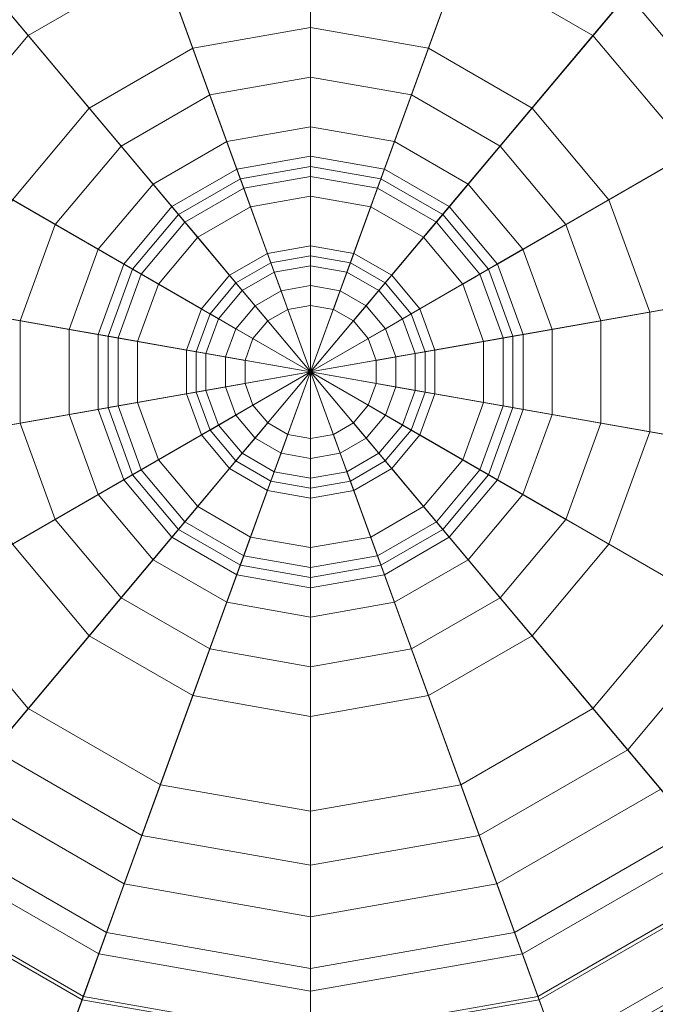
# Model space of a CAD drawing. Units: inches. Extents: x 375 to 1122, y 27 to 1069.
# Tile 129 of 155: x 721.601 to 722.65, y 901.45 to 903.075. Entities that reach past the tile are written whole.
import ezdxf

# ---------------------------------------------------------------- set-up
doc = ezdxf.new("R2010")
doc.units = ezdxf.units.IN
doc.layers.add('A-ANNO-DIMS', color=2, linetype='Continuous', lineweight=18)
doc.layers.add('Furniture', color=30, linetype='Continuous', lineweight=18)
doc.styles.get("Standard").update_dxf_attribs({"font": 'arial.ttf'})
doc.dimstyles.new('ISO-25', dxfattribs={"dimtxt": 12, "dimasz": 2.5, "dimexe": 1.5, "dimexo": 1.5, "dimtad": 1, "dimdec": 1, "dimlunit": 3, "dimtxsty": 'Standard', "dimblk": 'ARCHTICK', "dimcen": 2.5, "dimadec": 0, "dimazin": 0, "dimtfac": 1, "dimtdec": 1, "dimtmove": 0, "dimatfit": 3, "dimfxl": 1.5, "dimfxlon": 1, "dimarcsym": 0})

# ---------------------------------------------------------------- blocks, each defined once
blk = doc.blocks.new('A$C403C54AD')
for points in [[(0.889855, 0.961682, -0.042784), (0.895735, 0.928335, -0.039705), (0.895735, 0.928335, -0.039705), (0.878804, 0.95766, -0.042784)], [(0.901615, 0.961682, -0.042784), (0.895735, 0.928335, -0.039705), (0.895735, 0.928335, -0.039705), (0.889855, 0.961682, -0.042784)], [(0.912666, 0.95766, -0.042784), (0.895735, 0.928335, -0.039705), (0.895735, 0.928335, -0.039705), (0.901615, 0.961682, -0.042784)], [(0.893266, 0.942333, -0.036278), (0.890422, 0.958466, -0.039553), (0.880436, 0.954832, -0.039553), (0.888627, 0.940645, -0.036278)], [(0.898203, 0.942333, -0.036278), (0.901048, 0.958466, -0.039553), (0.890422, 0.958466, -0.039553), (0.893266, 0.942333, -0.036278)], [(0.902842, 0.940645, -0.036278), (0.911033, 0.954832, -0.039553), (0.901048, 0.958466, -0.039553), (0.898203, 0.942333, -0.036278)], [(0.878804, 0.95766, -0.042784), (0.895735, 0.928335, -0.039705), (0.895735, 0.928335, -0.039705), (0.869795, 0.950101, -0.042784)], [(0.921675, 0.950101, -0.042784), (0.895735, 0.928335, -0.039705), (0.895735, 0.928335, -0.039705), (0.912666, 0.95766, -0.042784)], [(0.888627, 0.940645, -0.036278), (0.880436, 0.954832, -0.039553), (0.872296, 0.948002, -0.039553), (0.884846, 0.937471, -0.036278)], [(0.906623, 0.937471, -0.036278), (0.919173, 0.948002, -0.039553), (0.911033, 0.954832, -0.039553), (0.902842, 0.940645, -0.036278)], [(0.882023, 0.952084, 0.060725), (0.885556, 0.945965, 0.050493), (0.88014, 0.94142, 0.050493), (0.874727, 0.945962, 0.060725)], [(0.916743, 0.945962, 0.060725), (0.911329, 0.94142, 0.050493), (0.905913, 0.945965, 0.050493), (0.909447, 0.952084, 0.060725)], [(0.869795, 0.950101, -0.042784), (0.895735, 0.928335, -0.039705), (0.895735, 0.928335, -0.039705), (0.863915, 0.939916, -0.042784)], [(0.927555, 0.939916, -0.042784), (0.895735, 0.928335, -0.039705), (0.895735, 0.928335, -0.039705), (0.921675, 0.950101, -0.042784)], [(0.924486, 0.938799, -0.039553), (0.927555, 0.939916, -0.042784), (0.921675, 0.950101, -0.042784), (0.919173, 0.948002, -0.039553)], [(0.886671, 0.944033, 0.05268), (0.883428, 0.94965, 0.062072), (0.87688, 0.944156, 0.062072), (0.881848, 0.939987, 0.05268)], [(0.909621, 0.939987, 0.05268), (0.914589, 0.944156, 0.062072), (0.908041, 0.94965, 0.062072), (0.904798, 0.944033, 0.05268)], [(0.924448, 0.938785, 0.1202), (0.92718, 0.93978, 0.106976), (0.921369, 0.949844, 0.106976), (0.919142, 0.947976, 0.1202)], [(0.92718, 0.93978, 0.106976), (0.926546, 0.939549, 0.078734), (0.920852, 0.949411, 0.078734), (0.921369, 0.949844, 0.106976)], [(0.926546, 0.939549, 0.078734), (0.921505, 0.937714, 0.060725), (0.916743, 0.945962, 0.060725), (0.920852, 0.949411, 0.078734)], [(0.884846, 0.937471, -0.036278), (0.872296, 0.948002, -0.039553), (0.866983, 0.938799, -0.039553), (0.882378, 0.933196, -0.036278)], [(0.8922, 0.948383, 0.050493), (0.893978, 0.9383, 0.043125), (0.890675, 0.937098, 0.043125), (0.885556, 0.945965, 0.050493)], [(0.89927, 0.948383, 0.050493), (0.897492, 0.9383, 0.043125), (0.893978, 0.9383, 0.043125), (0.8922, 0.948383, 0.050493)], [(0.905913, 0.945965, 0.050493), (0.900794, 0.937098, 0.043125), (0.897492, 0.9383, 0.043125), (0.89927, 0.948383, 0.050493)], [(0.909092, 0.933196, -0.036278), (0.924486, 0.938799, -0.039553), (0.919173, 0.948002, -0.039553), (0.906623, 0.937471, -0.036278)], [(0.919753, 0.937076, 0.129606), (0.924448, 0.938785, 0.1202), (0.919142, 0.947976, 0.1202), (0.915314, 0.944764, 0.129606)], [(0.924281, 0.938725, 0.106759), (0.921641, 0.937764, 0.119395), (0.916854, 0.946056, 0.119395), (0.919006, 0.947862, 0.106759)], [(0.923663, 0.9385, 0.079219), (0.924281, 0.938725, 0.106759), (0.919006, 0.947862, 0.106759), (0.918502, 0.947439, 0.079219)], [(0.918863, 0.936753, 0.062072), (0.923663, 0.9385, 0.079219), (0.918502, 0.947439, 0.079219), (0.914589, 0.944156, 0.062072)], [(0.894188, 0.937103, 0.046044), (0.892587, 0.946186, 0.05268), (0.886671, 0.944033, 0.05268), (0.891283, 0.936046, 0.046044)], [(0.897281, 0.937103, 0.046044), (0.898882, 0.946186, 0.05268), (0.892587, 0.946186, 0.05268), (0.894188, 0.937103, 0.046044)], [(0.900187, 0.936046, 0.046044), (0.904798, 0.944033, 0.05268), (0.898882, 0.946186, 0.05268), (0.897281, 0.937103, 0.046044)], [(0.921641, 0.937764, 0.119395), (0.91686, 0.936024, 0.129606), (0.912956, 0.942785, 0.129606), (0.916854, 0.946056, 0.119395)], [(0.885556, 0.945965, 0.050493), (0.890675, 0.937098, 0.043125), (0.887983, 0.934839, 0.043125), (0.88014, 0.94142, 0.050493)], [(0.911329, 0.94142, 0.050493), (0.903486, 0.934839, 0.043125), (0.900794, 0.937098, 0.043125), (0.905913, 0.945965, 0.050493)], [(0.921505, 0.937714, 0.060725), (0.914864, 0.935297, 0.050493), (0.911329, 0.94142, 0.050493), (0.916743, 0.945962, 0.060725)], [(0.91686, 0.936024, 0.129606), (0.919753, 0.937076, 0.129606), (0.915314, 0.944764, 0.129606), (0.912956, 0.942785, 0.129606)], [(0.881848, 0.939987, 0.05268), (0.87688, 0.944156, 0.062072), (0.872606, 0.936753, 0.062072), (0.878701, 0.934534, 0.05268)], [(0.891283, 0.936046, 0.046044), (0.886671, 0.944033, 0.05268), (0.881848, 0.939987, 0.05268), (0.888914, 0.934058, 0.046044)], [(0.902556, 0.934058, 0.046044), (0.909621, 0.939987, 0.05268), (0.904798, 0.944033, 0.05268), (0.900187, 0.936046, 0.046044)], [(0.912769, 0.934534, 0.05268), (0.918863, 0.936753, 0.062072), (0.914589, 0.944156, 0.062072), (0.909621, 0.939987, 0.05268)], [(0.893622, 0.940316, -0.033413), (0.893266, 0.942333, -0.036278), (0.888627, 0.940645, -0.036278), (0.889651, 0.938871, -0.033413)], [(0.897847, 0.940316, -0.033413), (0.898203, 0.942333, -0.036278), (0.893266, 0.942333, -0.036278), (0.893622, 0.940316, -0.033413)], [(0.901818, 0.938871, -0.033413), (0.902842, 0.940645, -0.036278), (0.898203, 0.942333, -0.036278), (0.897847, 0.940316, -0.033413)], [(0.88014, 0.94142, 0.050493), (0.887983, 0.934839, 0.043125), (0.886226, 0.931795, 0.043125), (0.876605, 0.935297, 0.050493)], [(0.914864, 0.935297, 0.050493), (0.905243, 0.931795, 0.043125), (0.903486, 0.934839, 0.043125), (0.911329, 0.94142, 0.050493)], [(0.889651, 0.938871, -0.033413), (0.888627, 0.940645, -0.036278), (0.884846, 0.937471, -0.036278), (0.886415, 0.936155, -0.033413)], [(0.894333, 0.936283, -0.031367), (0.893622, 0.940316, -0.033413), (0.889651, 0.938871, -0.033413), (0.891699, 0.935324, -0.031367)], [(0.897136, 0.936283, -0.031367), (0.897847, 0.940316, -0.033413), (0.893622, 0.940316, -0.033413), (0.894333, 0.936283, -0.031367)], [(0.89977, 0.935324, -0.031367), (0.901818, 0.938871, -0.033413), (0.897847, 0.940316, -0.033413), (0.897136, 0.936283, -0.031367)], [(0.905055, 0.936155, -0.033413), (0.906623, 0.937471, -0.036278), (0.902842, 0.940645, -0.036278), (0.901818, 0.938871, -0.033413)], [(0.863915, 0.939916, -0.042784), (0.895735, 0.928335, -0.039705), (0.895735, 0.928335, -0.039705), (0.861872, 0.928335, -0.042784)], [(0.888914, 0.934058, 0.046044), (0.881848, 0.939987, 0.05268), (0.878701, 0.934534, 0.05268), (0.887368, 0.93138, 0.046044)], [(0.929597, 0.928335, -0.042784), (0.895735, 0.928335, -0.039705), (0.895735, 0.928335, -0.039705), (0.927555, 0.939916, -0.042784)], [(0.904102, 0.93138, 0.046044), (0.912769, 0.934534, 0.05268), (0.909621, 0.939987, 0.05268), (0.902556, 0.934058, 0.046044)], [(0.928523, 0.928335, 0.078734), (0.923158, 0.928335, 0.060725), (0.921505, 0.937714, 0.060725), (0.926546, 0.939549, 0.078734)], [(0.882378, 0.933196, -0.036278), (0.866983, 0.938799, -0.039553), (0.865138, 0.928335, -0.039553), (0.88152, 0.928335, -0.036278)], [(0.891699, 0.935324, -0.031367), (0.889651, 0.938871, -0.033413), (0.886415, 0.936155, -0.033413), (0.889552, 0.933523, -0.031367)], [(0.901917, 0.933523, -0.031367), (0.905055, 0.936155, -0.033413), (0.901818, 0.938871, -0.033413), (0.89977, 0.935324, -0.031367)], [(0.909949, 0.928335, -0.036278), (0.926331, 0.928335, -0.039553), (0.924486, 0.938799, -0.039553), (0.909092, 0.933196, -0.036278)], [(0.921294, 0.928335, 0.129606), (0.926291, 0.928335, 0.1202), (0.924448, 0.938785, 0.1202), (0.919753, 0.937076, 0.129606)], [(0.926113, 0.928335, 0.106759), (0.923304, 0.928335, 0.119395), (0.921641, 0.937764, 0.119395), (0.924281, 0.938725, 0.106759)], [(0.893978, 0.9383, 0.043125), (0.894831, 0.93346, 0.042307), (0.893133, 0.932841, 0.042307), (0.890675, 0.937098, 0.043125)], [(0.897492, 0.9383, 0.043125), (0.896638, 0.93346, 0.042307), (0.894831, 0.93346, 0.042307), (0.893978, 0.9383, 0.043125)], [(0.900794, 0.937098, 0.043125), (0.898337, 0.932841, 0.042307), (0.896638, 0.93346, 0.042307), (0.897492, 0.9383, 0.043125)], [(0.920348, 0.928335, 0.062072), (0.925455, 0.928335, 0.079219), (0.923663, 0.9385, 0.079219), (0.918863, 0.936753, 0.062072)], [(0.886415, 0.936155, -0.033413), (0.884846, 0.937471, -0.036278), (0.882378, 0.933196, -0.036278), (0.884302, 0.932496, -0.033413)], [(0.907167, 0.932496, -0.033413), (0.909092, 0.933196, -0.036278), (0.906623, 0.937471, -0.036278), (0.905055, 0.936155, -0.033413)], [(0.923158, 0.928335, 0.060725), (0.916092, 0.928335, 0.050493), (0.914864, 0.935297, 0.050493), (0.921505, 0.937714, 0.060725)], [(0.923304, 0.928335, 0.119395), (0.918216, 0.928335, 0.129606), (0.91686, 0.936024, 0.129606), (0.921641, 0.937764, 0.119395)], [(0.890675, 0.937098, 0.043125), (0.893133, 0.932841, 0.042307), (0.891748, 0.93168, 0.042307), (0.887983, 0.934839, 0.043125)], [(0.895735, 0.928335, 0.044561), (0.894188, 0.937103, 0.046044), (0.891283, 0.936046, 0.046044), (0.895735, 0.928335, 0.044561)], [(0.895735, 0.928335, 0.044561), (0.897281, 0.937103, 0.046044), (0.894188, 0.937103, 0.046044), (0.895735, 0.928335, 0.044561)], [(0.895735, 0.928335, 0.044561), (0.900187, 0.936046, 0.046044), (0.897281, 0.937103, 0.046044), (0.895735, 0.928335, 0.044561)], [(0.903486, 0.934839, 0.043125), (0.899721, 0.93168, 0.042307), (0.898337, 0.932841, 0.042307), (0.900794, 0.937098, 0.043125)], [(0.918216, 0.928335, 0.129606), (0.921294, 0.928335, 0.129606), (0.919753, 0.937076, 0.129606), (0.91686, 0.936024, 0.129606)], [(0.894475, 0.935476, 0.041488), (0.894262, 0.936686, 0.039442), (0.891494, 0.935679, 0.039442), (0.892109, 0.934615, 0.041488)], [(0.894262, 0.936686, 0.039442), (0.894973, 0.932653, 0.037395), (0.893542, 0.932132, 0.037395), (0.891494, 0.935679, 0.039442)], [(0.896994, 0.935476, 0.041488), (0.897207, 0.936686, 0.039442), (0.894262, 0.936686, 0.039442), (0.894475, 0.935476, 0.041488)], [(0.897207, 0.936686, 0.039442), (0.896496, 0.932653, 0.037395), (0.894973, 0.932653, 0.037395), (0.894262, 0.936686, 0.039442)], [(0.899975, 0.935679, 0.039442), (0.897927, 0.932132, 0.037395), (0.896496, 0.932653, 0.037395), (0.897207, 0.936686, 0.039442)], [(0.899361, 0.934615, 0.041488), (0.899975, 0.935679, 0.039442), (0.897207, 0.936686, 0.039442), (0.896994, 0.935476, 0.041488)], [(0.913862, 0.928335, 0.05268), (0.920348, 0.928335, 0.062072), (0.918863, 0.936753, 0.062072), (0.912769, 0.934534, 0.05268)], [(0.894902, 0.933056, -0.026046), (0.894333, 0.936283, -0.031367), (0.891699, 0.935324, -0.031367), (0.893337, 0.932487, -0.026046)], [(0.896567, 0.933056, -0.026046), (0.897136, 0.936283, -0.031367), (0.894333, 0.936283, -0.031367), (0.894902, 0.933056, -0.026046)], [(0.898132, 0.932487, -0.026046), (0.89977, 0.935324, -0.031367), (0.897136, 0.936283, -0.031367), (0.896567, 0.933056, -0.026046)], [(0.889552, 0.933523, -0.031367), (0.886415, 0.936155, -0.033413), (0.884302, 0.932496, -0.033413), (0.88815, 0.931095, -0.031367)], [(0.895735, 0.928335, 0.044561), (0.891283, 0.936046, 0.046044), (0.888914, 0.934058, 0.046044), (0.895735, 0.928335, 0.044561)], [(0.895735, 0.928335, 0.044561), (0.902556, 0.934058, 0.046044), (0.900187, 0.936046, 0.046044), (0.895735, 0.928335, 0.044561)], [(0.903319, 0.931095, -0.031367), (0.907167, 0.932496, -0.033413), (0.905055, 0.936155, -0.033413), (0.901917, 0.933523, -0.031367)], [(0.891494, 0.935679, 0.039442), (0.893542, 0.932132, 0.037395), (0.892376, 0.931153, 0.037395), (0.889238, 0.933786, 0.039442)], [(0.892109, 0.934615, 0.041488), (0.891494, 0.935679, 0.039442), (0.889238, 0.933786, 0.039442), (0.890179, 0.932996, 0.041488)], [(0.894831, 0.93346, 0.042307), (0.894475, 0.935476, 0.041488), (0.892109, 0.934615, 0.041488), (0.893133, 0.932841, 0.042307)], [(0.896638, 0.93346, 0.042307), (0.896994, 0.935476, 0.041488), (0.894475, 0.935476, 0.041488), (0.894831, 0.93346, 0.042307)], [(0.898337, 0.932841, 0.042307), (0.899361, 0.934615, 0.041488), (0.896994, 0.935476, 0.041488), (0.896638, 0.93346, 0.042307)], [(0.902231, 0.933786, 0.039442), (0.899094, 0.931153, 0.037395), (0.897927, 0.932132, 0.037395), (0.899975, 0.935679, 0.039442)], [(0.90129, 0.932996, 0.041488), (0.902231, 0.933786, 0.039442), (0.899975, 0.935679, 0.039442), (0.899361, 0.934615, 0.041488)], [(0.876605, 0.935297, 0.050493), (0.886226, 0.931795, 0.043125), (0.885616, 0.928335, 0.043125), (0.875377, 0.928335, 0.050493)], [(0.893337, 0.932487, -0.026046), (0.891699, 0.935324, -0.031367), (0.889552, 0.933523, -0.031367), (0.892062, 0.931416, -0.026046)], [(0.899407, 0.931416, -0.026046), (0.901917, 0.933523, -0.031367), (0.89977, 0.935324, -0.031367), (0.898132, 0.932487, -0.026046)], [(0.916092, 0.928335, 0.050493), (0.905853, 0.928335, 0.043125), (0.905243, 0.931795, 0.043125), (0.914864, 0.935297, 0.050493)], [(0.887983, 0.934839, 0.043125), (0.891748, 0.93168, 0.042307), (0.890844, 0.930114, 0.042307), (0.886226, 0.931795, 0.043125)], [(0.893133, 0.932841, 0.042307), (0.892109, 0.934615, 0.041488), (0.890179, 0.932996, 0.041488), (0.891748, 0.93168, 0.042307)], [(0.899721, 0.93168, 0.042307), (0.90129, 0.932996, 0.041488), (0.899361, 0.934615, 0.041488), (0.898337, 0.932841, 0.042307)], [(0.905243, 0.931795, 0.043125), (0.900625, 0.930114, 0.042307), (0.899721, 0.93168, 0.042307), (0.903486, 0.934839, 0.043125)], [(0.887368, 0.93138, 0.046044), (0.878701, 0.934534, 0.05268), (0.877607, 0.928335, 0.05268), (0.886831, 0.928335, 0.046044)], [(0.904639, 0.928335, 0.046044), (0.913862, 0.928335, 0.05268), (0.912769, 0.934534, 0.05268), (0.904102, 0.93138, 0.046044)], [(0.895735, 0.928335, 0.044561), (0.888914, 0.934058, 0.046044), (0.887368, 0.93138, 0.046044), (0.895735, 0.928335, 0.044561)], [(0.889238, 0.933786, 0.039442), (0.892376, 0.931153, 0.037395), (0.891614, 0.929834, 0.037395), (0.887766, 0.931235, 0.039442)], [(0.890179, 0.932996, 0.041488), (0.889238, 0.933786, 0.039442), (0.887766, 0.931235, 0.039442), (0.88892, 0.930815, 0.041488)], [(0.895735, 0.928335, 0.044561), (0.904102, 0.93138, 0.046044), (0.902556, 0.934058, 0.046044), (0.895735, 0.928335, 0.044561)], [(0.903704, 0.931235, 0.039442), (0.899855, 0.929834, 0.037395), (0.899094, 0.931153, 0.037395), (0.902231, 0.933786, 0.039442)], [(0.902549, 0.930815, 0.041488), (0.903704, 0.931235, 0.039442), (0.902231, 0.933786, 0.039442), (0.90129, 0.932996, 0.041488)], [(0.892062, 0.931416, -0.026046), (0.889552, 0.933523, -0.031367), (0.88815, 0.931095, -0.031367), (0.891229, 0.929974, -0.026046)], [(0.90024, 0.929974, -0.026046), (0.903319, 0.931095, -0.031367), (0.901917, 0.933523, -0.031367), (0.899407, 0.931416, -0.026046)], [(0.884302, 0.932496, -0.033413), (0.882378, 0.933196, -0.036278), (0.88152, 0.928335, -0.036278), (0.883568, 0.928335, -0.033413)], [(0.891748, 0.93168, 0.042307), (0.890179, 0.932996, 0.041488), (0.88892, 0.930815, 0.041488), (0.890844, 0.930114, 0.042307)], [(0.895115, 0.931846, -0.017451), (0.894902, 0.933056, -0.026046), (0.893337, 0.932487, -0.026046), (0.893952, 0.931423, -0.017451)], [(0.896354, 0.931846, -0.017451), (0.896567, 0.933056, -0.026046), (0.894902, 0.933056, -0.026046), (0.895115, 0.931846, -0.017451)], [(0.897518, 0.931423, -0.017451), (0.898132, 0.932487, -0.026046), (0.896567, 0.933056, -0.026046), (0.896354, 0.931846, -0.017451)], [(0.900625, 0.930114, 0.042307), (0.902549, 0.930815, 0.041488), (0.90129, 0.932996, 0.041488), (0.899721, 0.93168, 0.042307)], [(0.907901, 0.928335, -0.033413), (0.909949, 0.928335, -0.036278), (0.909092, 0.933196, -0.036278), (0.907167, 0.932496, -0.033413)], [(0.894973, 0.932653, 0.037395), (0.895258, 0.93104, 0.030847), (0.894361, 0.930713, 0.030847), (0.893542, 0.932132, 0.037395)], [(0.896496, 0.932653, 0.037395), (0.896212, 0.93104, 0.030847), (0.895258, 0.93104, 0.030847), (0.894973, 0.932653, 0.037395)], [(0.897927, 0.932132, 0.037395), (0.897108, 0.930713, 0.030847), (0.896212, 0.93104, 0.030847), (0.896496, 0.932653, 0.037395)], [(0.88815, 0.931095, -0.031367), (0.884302, 0.932496, -0.033413), (0.883568, 0.928335, -0.033413), (0.887664, 0.928335, -0.031367)], [(0.893952, 0.931423, -0.017451), (0.893337, 0.932487, -0.026046), (0.892062, 0.931416, -0.026046), (0.893003, 0.930627, -0.017451)], [(0.898466, 0.930627, -0.017451), (0.899407, 0.931416, -0.026046), (0.898132, 0.932487, -0.026046), (0.897518, 0.931423, -0.017451)], [(0.903806, 0.928335, -0.031367), (0.907901, 0.928335, -0.033413), (0.907167, 0.932496, -0.033413), (0.903319, 0.931095, -0.031367)], [(0.886226, 0.931795, 0.043125), (0.890844, 0.930114, 0.042307), (0.890531, 0.928335, 0.042307), (0.885616, 0.928335, 0.043125)], [(0.893542, 0.932132, 0.037395), (0.894361, 0.930713, 0.030847), (0.89363, 0.9301, 0.030847), (0.892376, 0.931153, 0.037395)], [(0.895258, 0.93104, 0.030847), (0.895115, 0.931846, -0.017451), (0.893952, 0.931423, -0.017451), (0.894361, 0.930713, 0.030847)], [(0.896212, 0.93104, 0.030847), (0.896354, 0.931846, -0.017451), (0.895115, 0.931846, -0.017451), (0.895258, 0.93104, 0.030847)], [(0.897108, 0.930713, 0.030847), (0.897518, 0.931423, -0.017451), (0.896354, 0.931846, -0.017451), (0.896212, 0.93104, 0.030847)], [(0.899094, 0.931153, 0.037395), (0.897839, 0.9301, 0.030847), (0.897108, 0.930713, 0.030847), (0.897927, 0.932132, 0.037395)], [(0.905853, 0.928335, 0.043125), (0.900939, 0.928335, 0.042307), (0.900625, 0.930114, 0.042307), (0.905243, 0.931795, 0.043125)], [(0.895735, 0.928335, 0.044561), (0.887368, 0.93138, 0.046044), (0.886831, 0.928335, 0.046044), (0.895735, 0.928335, 0.044561)], [(0.893003, 0.930627, -0.017451), (0.892062, 0.931416, -0.026046), (0.891229, 0.929974, -0.026046), (0.892384, 0.929554, -0.017451)], [(0.894361, 0.930713, 0.030847), (0.893952, 0.931423, -0.017451), (0.893003, 0.930627, -0.017451), (0.89363, 0.9301, 0.030847)], [(0.895735, 0.928335, 0.044561), (0.904639, 0.928335, 0.046044), (0.904102, 0.93138, 0.046044), (0.895735, 0.928335, 0.044561)], [(0.897839, 0.9301, 0.030847), (0.898466, 0.930627, -0.017451), (0.897518, 0.931423, -0.017451), (0.897108, 0.930713, 0.030847)], [(0.899085, 0.929554, -0.017451), (0.90024, 0.929974, -0.026046), (0.899407, 0.931416, -0.026046), (0.898466, 0.930627, -0.017451)], [(0.887766, 0.931235, 0.039442), (0.891614, 0.929834, 0.037395), (0.89135, 0.928335, 0.037395), (0.887254, 0.928335, 0.039442)], [(0.88892, 0.930815, 0.041488), (0.887766, 0.931235, 0.039442), (0.887254, 0.928335, 0.039442), (0.888483, 0.928335, 0.041488)], [(0.891229, 0.929974, -0.026046), (0.88815, 0.931095, -0.031367), (0.887664, 0.928335, -0.031367), (0.89094, 0.928335, -0.026046)], [(0.892376, 0.931153, 0.037395), (0.89363, 0.9301, 0.030847), (0.893153, 0.929274, 0.030847), (0.891614, 0.929834, 0.037395)], [(0.899855, 0.929834, 0.037395), (0.898316, 0.929274, 0.030847), (0.897839, 0.9301, 0.030847), (0.899094, 0.931153, 0.037395)], [(0.904215, 0.928335, 0.039442), (0.90012, 0.928335, 0.037395), (0.899855, 0.929834, 0.037395), (0.903704, 0.931235, 0.039442)], [(0.900529, 0.928335, -0.026046), (0.903806, 0.928335, -0.031367), (0.903319, 0.931095, -0.031367), (0.90024, 0.929974, -0.026046)], [(0.902987, 0.928335, 0.041488), (0.904215, 0.928335, 0.039442), (0.903704, 0.931235, 0.039442), (0.902549, 0.930815, 0.041488)], [(0.890844, 0.930114, 0.042307), (0.88892, 0.930815, 0.041488), (0.888483, 0.928335, 0.041488), (0.890531, 0.928335, 0.042307)], [(0.89363, 0.9301, 0.030847), (0.893003, 0.930627, -0.017451), (0.892384, 0.929554, -0.017451), (0.893153, 0.929274, 0.030847)], [(0.898316, 0.929274, 0.030847), (0.899085, 0.929554, -0.017451), (0.898466, 0.930627, -0.017451), (0.897839, 0.9301, 0.030847)], [(0.900939, 0.928335, 0.042307), (0.902987, 0.928335, 0.041488), (0.902549, 0.930815, 0.041488), (0.900625, 0.930114, 0.042307)], [(0.892384, 0.929554, -0.017451), (0.891229, 0.929974, -0.026046), (0.89094, 0.928335, -0.026046), (0.892169, 0.928335, -0.017451)], [(0.891614, 0.929834, 0.037395), (0.893153, 0.929274, 0.030847), (0.892988, 0.928335, 0.030847), (0.89135, 0.928335, 0.037395)], [(0.90012, 0.928335, 0.037395), (0.898481, 0.928335, 0.030847), (0.898316, 0.929274, 0.030847), (0.899855, 0.929834, 0.037395)], [(0.899301, 0.928335, -0.017451), (0.900529, 0.928335, -0.026046), (0.90024, 0.929974, -0.026046), (0.899085, 0.929554, -0.017451)], [(0.893153, 0.929274, 0.030847), (0.892384, 0.929554, -0.017451), (0.892169, 0.928335, -0.017451), (0.892988, 0.928335, 0.030847)], [(0.898481, 0.928335, 0.030847), (0.899301, 0.928335, -0.017451), (0.899085, 0.929554, -0.017451), (0.898316, 0.929274, 0.030847)], [(0.861872, 0.928335, -0.042784), (0.895735, 0.928335, -0.039705), (0.895735, 0.928335, -0.039705), (0.863915, 0.916753, -0.042784)], [(0.863915, 0.916753, -0.042784), (0.895735, 0.928335, -0.039705), (0.895735, 0.928335, -0.039705), (0.869795, 0.906568, -0.042784)], [(0.88152, 0.928335, -0.036278), (0.865138, 0.928335, -0.039553), (0.866983, 0.91787, -0.039553), (0.882378, 0.923473, -0.036278)], [(0.869795, 0.906568, -0.042784), (0.895735, 0.928335, -0.039705), (0.895735, 0.928335, -0.039705), (0.878804, 0.899009, -0.042784)], [(0.875377, 0.928335, 0.050493), (0.885616, 0.928335, 0.043125), (0.886226, 0.924874, 0.043125), (0.876605, 0.921372, 0.050493)], [(0.886831, 0.928335, 0.046044), (0.877607, 0.928335, 0.05268), (0.878701, 0.922135, 0.05268), (0.887368, 0.925289, 0.046044)], [(0.878804, 0.899009, -0.042784), (0.895735, 0.928335, -0.039705), (0.895735, 0.928335, -0.039705), (0.889855, 0.894987, -0.042784)], [(0.883568, 0.928335, -0.033413), (0.88152, 0.928335, -0.036278), (0.882378, 0.923473, -0.036278), (0.884302, 0.924173, -0.033413)], [(0.887664, 0.928335, -0.031367), (0.883568, 0.928335, -0.033413), (0.884302, 0.924173, -0.033413), (0.88815, 0.925574, -0.031367)], [(0.885616, 0.928335, 0.043125), (0.890531, 0.928335, 0.042307), (0.890844, 0.926555, 0.042307), (0.886226, 0.924874, 0.043125)], [(0.895735, 0.928335, 0.044561), (0.886831, 0.928335, 0.046044), (0.887368, 0.925289, 0.046044), (0.895735, 0.928335, 0.044561)], [(0.887254, 0.928335, 0.039442), (0.89135, 0.928335, 0.037395), (0.891614, 0.926835, 0.037395), (0.887766, 0.925434, 0.039442)], [(0.888483, 0.928335, 0.041488), (0.887254, 0.928335, 0.039442), (0.887766, 0.925434, 0.039442), (0.88892, 0.925854, 0.041488)], [(0.895735, 0.928335, 0.044561), (0.887368, 0.925289, 0.046044), (0.888914, 0.922611, 0.046044), (0.895735, 0.928335, 0.044561)], [(0.89094, 0.928335, -0.026046), (0.887664, 0.928335, -0.031367), (0.88815, 0.925574, -0.031367), (0.891229, 0.926695, -0.026046)], [(0.890531, 0.928335, 0.042307), (0.888483, 0.928335, 0.041488), (0.88892, 0.925854, 0.041488), (0.890844, 0.926555, 0.042307)], [(0.895735, 0.928335, 0.044561), (0.888914, 0.922611, 0.046044), (0.891283, 0.920623, 0.046044), (0.895735, 0.928335, 0.044561)], [(0.889855, 0.894987, -0.042784), (0.895735, 0.928335, -0.039705), (0.895735, 0.928335, -0.039705), (0.901615, 0.894987, -0.042784)], [(0.892169, 0.928335, -0.017451), (0.89094, 0.928335, -0.026046), (0.891229, 0.926695, -0.026046), (0.892384, 0.927115, -0.017451)], [(0.895735, 0.928335, 0.044561), (0.891283, 0.920623, 0.046044), (0.894188, 0.919566, 0.046044), (0.895735, 0.928335, 0.044561)], [(0.89135, 0.928335, 0.037395), (0.892988, 0.928335, 0.030847), (0.893153, 0.927395, 0.030847), (0.891614, 0.926835, 0.037395)], [(0.892988, 0.928335, 0.030847), (0.892169, 0.928335, -0.017451), (0.892384, 0.927115, -0.017451), (0.893153, 0.927395, 0.030847)], [(0.895735, 0.928335, 0.044561), (0.894188, 0.919566, 0.046044), (0.897281, 0.919566, 0.046044), (0.895735, 0.928335, 0.044561)], [(0.895735, 0.928335, 0.044561), (0.904102, 0.925289, 0.046044), (0.904639, 0.928335, 0.046044), (0.895735, 0.928335, 0.044561)], [(0.895735, 0.928335, 0.044561), (0.902556, 0.922611, 0.046044), (0.904102, 0.925289, 0.046044), (0.895735, 0.928335, 0.044561)], [(0.895735, 0.928335, 0.044561), (0.900187, 0.920623, 0.046044), (0.902556, 0.922611, 0.046044), (0.895735, 0.928335, 0.044561)], [(0.895735, 0.928335, 0.044561), (0.897281, 0.919566, 0.046044), (0.900187, 0.920623, 0.046044), (0.895735, 0.928335, 0.044561)], [(0.927555, 0.916753, -0.042784), (0.895735, 0.928335, -0.039705), (0.895735, 0.928335, -0.039705), (0.929597, 0.928335, -0.042784)], [(0.921675, 0.906568, -0.042784), (0.895735, 0.928335, -0.039705), (0.895735, 0.928335, -0.039705), (0.927555, 0.916753, -0.042784)], [(0.912666, 0.899009, -0.042784), (0.895735, 0.928335, -0.039705), (0.895735, 0.928335, -0.039705), (0.921675, 0.906568, -0.042784)], [(0.901615, 0.894987, -0.042784), (0.895735, 0.928335, -0.039705), (0.895735, 0.928335, -0.039705), (0.912666, 0.899009, -0.042784)], [(0.899855, 0.926835, 0.037395), (0.898316, 0.927395, 0.030847), (0.898481, 0.928335, 0.030847), (0.90012, 0.928335, 0.037395)], [(0.898316, 0.927395, 0.030847), (0.899085, 0.927115, -0.017451), (0.899301, 0.928335, -0.017451), (0.898481, 0.928335, 0.030847)], [(0.899085, 0.927115, -0.017451), (0.90024, 0.926695, -0.026046), (0.900529, 0.928335, -0.026046), (0.899301, 0.928335, -0.017451)], [(0.903704, 0.925434, 0.039442), (0.899855, 0.926835, 0.037395), (0.90012, 0.928335, 0.037395), (0.904215, 0.928335, 0.039442)], [(0.90024, 0.926695, -0.026046), (0.903319, 0.925574, -0.031367), (0.903806, 0.928335, -0.031367), (0.900529, 0.928335, -0.026046)], [(0.900625, 0.926555, 0.042307), (0.902549, 0.925854, 0.041488), (0.902987, 0.928335, 0.041488), (0.900939, 0.928335, 0.042307)], [(0.905243, 0.924874, 0.043125), (0.900625, 0.926555, 0.042307), (0.900939, 0.928335, 0.042307), (0.905853, 0.928335, 0.043125)], [(0.902549, 0.925854, 0.041488), (0.903704, 0.925434, 0.039442), (0.904215, 0.928335, 0.039442), (0.902987, 0.928335, 0.041488)], [(0.903319, 0.925574, -0.031367), (0.907167, 0.924173, -0.033413), (0.907901, 0.928335, -0.033413), (0.903806, 0.928335, -0.031367)], [(0.904102, 0.925289, 0.046044), (0.912769, 0.922135, 0.05268), (0.913862, 0.928335, 0.05268), (0.904639, 0.928335, 0.046044)], [(0.914864, 0.921372, 0.050493), (0.905243, 0.924874, 0.043125), (0.905853, 0.928335, 0.043125), (0.916092, 0.928335, 0.050493)], [(0.907167, 0.924173, -0.033413), (0.909092, 0.923473, -0.036278), (0.909949, 0.928335, -0.036278), (0.907901, 0.928335, -0.033413)], [(0.909092, 0.923473, -0.036278), (0.924486, 0.91787, -0.039553), (0.926331, 0.928335, -0.039553), (0.909949, 0.928335, -0.036278)], [(0.912769, 0.922135, 0.05268), (0.918863, 0.919916, 0.062072), (0.920348, 0.928335, 0.062072), (0.913862, 0.928335, 0.05268)], [(0.921505, 0.918955, 0.060725), (0.914864, 0.921372, 0.050493), (0.916092, 0.928335, 0.050493), (0.923158, 0.928335, 0.060725)], [(0.91686, 0.920646, 0.129606), (0.919753, 0.919593, 0.129606), (0.921294, 0.928335, 0.129606), (0.918216, 0.928335, 0.129606)], [(0.921641, 0.918905, 0.119395), (0.91686, 0.920646, 0.129606), (0.918216, 0.928335, 0.129606), (0.923304, 0.928335, 0.119395)], [(0.918863, 0.919916, 0.062072), (0.923663, 0.918169, 0.079219), (0.925455, 0.928335, 0.079219), (0.920348, 0.928335, 0.062072)], [(0.919753, 0.919593, 0.129606), (0.924448, 0.917884, 0.1202), (0.926291, 0.928335, 0.1202), (0.921294, 0.928335, 0.129606)], [(0.926546, 0.91712, 0.078734), (0.921505, 0.918955, 0.060725), (0.923158, 0.928335, 0.060725), (0.928523, 0.928335, 0.078734)], [(0.924281, 0.917944, 0.106759), (0.921641, 0.918905, 0.119395), (0.923304, 0.928335, 0.119395), (0.926113, 0.928335, 0.106759)], [(0.891614, 0.926835, 0.037395), (0.893153, 0.927395, 0.030847), (0.89363, 0.926569, 0.030847), (0.892376, 0.925516, 0.037395)], [(0.893153, 0.927395, 0.030847), (0.892384, 0.927115, -0.017451), (0.893003, 0.926042, -0.017451), (0.89363, 0.926569, 0.030847)], [(0.899094, 0.925516, 0.037395), (0.897839, 0.926569, 0.030847), (0.898316, 0.927395, 0.030847), (0.899855, 0.926835, 0.037395)], [(0.897839, 0.926569, 0.030847), (0.898466, 0.926042, -0.017451), (0.899085, 0.927115, -0.017451), (0.898316, 0.927395, 0.030847)], [(0.892384, 0.927115, -0.017451), (0.891229, 0.926695, -0.026046), (0.892062, 0.925253, -0.026046), (0.893003, 0.926042, -0.017451)], [(0.898466, 0.926042, -0.017451), (0.899407, 0.925253, -0.026046), (0.90024, 0.926695, -0.026046), (0.899085, 0.927115, -0.017451)], [(0.886226, 0.924874, 0.043125), (0.890844, 0.926555, 0.042307), (0.891748, 0.924989, 0.042307), (0.887983, 0.92183, 0.043125)], [(0.887766, 0.925434, 0.039442), (0.891614, 0.926835, 0.037395), (0.892376, 0.925516, 0.037395), (0.889238, 0.922883, 0.039442)], [(0.891229, 0.926695, -0.026046), (0.88815, 0.925574, -0.031367), (0.889552, 0.923147, -0.031367), (0.892062, 0.925253, -0.026046)], [(0.890844, 0.926555, 0.042307), (0.88892, 0.925854, 0.041488), (0.890179, 0.923673, 0.041488), (0.891748, 0.924989, 0.042307)], [(0.892376, 0.925516, 0.037395), (0.89363, 0.926569, 0.030847), (0.894361, 0.925956, 0.030847), (0.893542, 0.924537, 0.037395)], [(0.89363, 0.926569, 0.030847), (0.893003, 0.926042, -0.017451), (0.893952, 0.925246, -0.017451), (0.894361, 0.925956, 0.030847)], [(0.897927, 0.924537, 0.037395), (0.897108, 0.925956, 0.030847), (0.897839, 0.926569, 0.030847), (0.899094, 0.925516, 0.037395)], [(0.897108, 0.925956, 0.030847), (0.897518, 0.925246, -0.017451), (0.898466, 0.926042, -0.017451), (0.897839, 0.926569, 0.030847)], [(0.902231, 0.922883, 0.039442), (0.899094, 0.925516, 0.037395), (0.899855, 0.926835, 0.037395), (0.903704, 0.925434, 0.039442)], [(0.899407, 0.925253, -0.026046), (0.901917, 0.923147, -0.031367), (0.903319, 0.925574, -0.031367), (0.90024, 0.926695, -0.026046)], [(0.899721, 0.924989, 0.042307), (0.90129, 0.923673, 0.041488), (0.902549, 0.925854, 0.041488), (0.900625, 0.926555, 0.042307)], [(0.903486, 0.92183, 0.043125), (0.899721, 0.924989, 0.042307), (0.900625, 0.926555, 0.042307), (0.905243, 0.924874, 0.043125)], [(0.88892, 0.925854, 0.041488), (0.887766, 0.925434, 0.039442), (0.889238, 0.922883, 0.039442), (0.890179, 0.923673, 0.041488)], [(0.893003, 0.926042, -0.017451), (0.892062, 0.925253, -0.026046), (0.893337, 0.924182, -0.026046), (0.893952, 0.925246, -0.017451)], [(0.893542, 0.924537, 0.037395), (0.894361, 0.925956, 0.030847), (0.895258, 0.92563, 0.030847), (0.894973, 0.924016, 0.037395)], [(0.894361, 0.925956, 0.030847), (0.893952, 0.925246, -0.017451), (0.895115, 0.924823, -0.017451), (0.895258, 0.92563, 0.030847)], [(0.896496, 0.924016, 0.037395), (0.896212, 0.92563, 0.030847), (0.897108, 0.925956, 0.030847), (0.897927, 0.924537, 0.037395)], [(0.896212, 0.92563, 0.030847), (0.896354, 0.924823, -0.017451), (0.897518, 0.925246, -0.017451), (0.897108, 0.925956, 0.030847)], [(0.897518, 0.925246, -0.017451), (0.898132, 0.924182, -0.026046), (0.899407, 0.925253, -0.026046), (0.898466, 0.926042, -0.017451)], [(0.90129, 0.923673, 0.041488), (0.902231, 0.922883, 0.039442), (0.903704, 0.925434, 0.039442), (0.902549, 0.925854, 0.041488)], [(0.887368, 0.925289, 0.046044), (0.878701, 0.922135, 0.05268), (0.881848, 0.916683, 0.05268), (0.888914, 0.922611, 0.046044)], [(0.88815, 0.925574, -0.031367), (0.884302, 0.924173, -0.033413), (0.886415, 0.920514, -0.033413), (0.889552, 0.923147, -0.031367)], [(0.889238, 0.922883, 0.039442), (0.892376, 0.925516, 0.037395), (0.893542, 0.924537, 0.037395), (0.891494, 0.92099, 0.039442)], [(0.892062, 0.925253, -0.026046), (0.889552, 0.923147, -0.031367), (0.891699, 0.921345, -0.031367), (0.893337, 0.924182, -0.026046)], [(0.893952, 0.925246, -0.017451), (0.893337, 0.924182, -0.026046), (0.894902, 0.923613, -0.026046), (0.895115, 0.924823, -0.017451)], [(0.894973, 0.924016, 0.037395), (0.895258, 0.92563, 0.030847), (0.896212, 0.92563, 0.030847), (0.896496, 0.924016, 0.037395)], [(0.895258, 0.92563, 0.030847), (0.895115, 0.924823, -0.017451), (0.896354, 0.924823, -0.017451), (0.896212, 0.92563, 0.030847)], [(0.896354, 0.924823, -0.017451), (0.896567, 0.923613, -0.026046), (0.898132, 0.924182, -0.026046), (0.897518, 0.925246, -0.017451)], [(0.899975, 0.92099, 0.039442), (0.897927, 0.924537, 0.037395), (0.899094, 0.925516, 0.037395), (0.902231, 0.922883, 0.039442)], [(0.898132, 0.924182, -0.026046), (0.89977, 0.921345, -0.031367), (0.901917, 0.923147, -0.031367), (0.899407, 0.925253, -0.026046)], [(0.901917, 0.923147, -0.031367), (0.905055, 0.920514, -0.033413), (0.907167, 0.924173, -0.033413), (0.903319, 0.925574, -0.031367)], [(0.902556, 0.922611, 0.046044), (0.909621, 0.916683, 0.05268), (0.912769, 0.922135, 0.05268), (0.904102, 0.925289, 0.046044)], [(0.876605, 0.921372, 0.050493), (0.886226, 0.924874, 0.043125), (0.887983, 0.92183, 0.043125), (0.88014, 0.915249, 0.050493)], [(0.887983, 0.92183, 0.043125), (0.891748, 0.924989, 0.042307), (0.893133, 0.923828, 0.042307), (0.890675, 0.919571, 0.043125)], [(0.891748, 0.924989, 0.042307), (0.890179, 0.923673, 0.041488), (0.892109, 0.922054, 0.041488), (0.893133, 0.923828, 0.042307)], [(0.898337, 0.923828, 0.042307), (0.899361, 0.922054, 0.041488), (0.90129, 0.923673, 0.041488), (0.899721, 0.924989, 0.042307)], [(0.900794, 0.919571, 0.043125), (0.898337, 0.923828, 0.042307), (0.899721, 0.924989, 0.042307), (0.903486, 0.92183, 0.043125)], [(0.911329, 0.915249, 0.050493), (0.903486, 0.92183, 0.043125), (0.905243, 0.924874, 0.043125), (0.914864, 0.921372, 0.050493)], [(0.891494, 0.92099, 0.039442), (0.893542, 0.924537, 0.037395), (0.894973, 0.924016, 0.037395), (0.894262, 0.919983, 0.039442)], [(0.895115, 0.924823, -0.017451), (0.894902, 0.923613, -0.026046), (0.896567, 0.923613, -0.026046), (0.896354, 0.924823, -0.017451)], [(0.897207, 0.919983, 0.039442), (0.896496, 0.924016, 0.037395), (0.897927, 0.924537, 0.037395), (0.899975, 0.92099, 0.039442)], [(0.884302, 0.924173, -0.033413), (0.882378, 0.923473, -0.036278), (0.884846, 0.919198, -0.036278), (0.886415, 0.920514, -0.033413)], [(0.893337, 0.924182, -0.026046), (0.891699, 0.921345, -0.031367), (0.894333, 0.920386, -0.031367), (0.894902, 0.923613, -0.026046)], [(0.896567, 0.923613, -0.026046), (0.897136, 0.920386, -0.031367), (0.89977, 0.921345, -0.031367), (0.898132, 0.924182, -0.026046)], [(0.905055, 0.920514, -0.033413), (0.906623, 0.919198, -0.036278), (0.909092, 0.923473, -0.036278), (0.907167, 0.924173, -0.033413)], [(0.890179, 0.923673, 0.041488), (0.889238, 0.922883, 0.039442), (0.891494, 0.92099, 0.039442), (0.892109, 0.922054, 0.041488)], [(0.890675, 0.919571, 0.043125), (0.893133, 0.923828, 0.042307), (0.894831, 0.92321, 0.042307), (0.893978, 0.91837, 0.043125)], [(0.893133, 0.923828, 0.042307), (0.892109, 0.922054, 0.041488), (0.894475, 0.921193, 0.041488), (0.894831, 0.92321, 0.042307)], [(0.894262, 0.919983, 0.039442), (0.894973, 0.924016, 0.037395), (0.896496, 0.924016, 0.037395), (0.897207, 0.919983, 0.039442)], [(0.896638, 0.92321, 0.042307), (0.896994, 0.921193, 0.041488), (0.899361, 0.922054, 0.041488), (0.898337, 0.923828, 0.042307)], [(0.897492, 0.91837, 0.043125), (0.896638, 0.92321, 0.042307), (0.898337, 0.923828, 0.042307), (0.900794, 0.919571, 0.043125)], [(0.899361, 0.922054, 0.041488), (0.899975, 0.92099, 0.039442), (0.902231, 0.922883, 0.039442), (0.90129, 0.923673, 0.041488)], [(0.882378, 0.923473, -0.036278), (0.866983, 0.91787, -0.039553), (0.872296, 0.908668, -0.039553), (0.884846, 0.919198, -0.036278)], [(0.894902, 0.923613, -0.026046), (0.894333, 0.920386, -0.031367), (0.897136, 0.920386, -0.031367), (0.896567, 0.923613, -0.026046)], [(0.906623, 0.919198, -0.036278), (0.919173, 0.908668, -0.039553), (0.924486, 0.91787, -0.039553), (0.909092, 0.923473, -0.036278)], [(0.889552, 0.923147, -0.031367), (0.886415, 0.920514, -0.033413), (0.889651, 0.917798, -0.033413), (0.891699, 0.921345, -0.031367)], [(0.893978, 0.91837, 0.043125), (0.894831, 0.92321, 0.042307), (0.896638, 0.92321, 0.042307), (0.897492, 0.91837, 0.043125)], [(0.894831, 0.92321, 0.042307), (0.894475, 0.921193, 0.041488), (0.896994, 0.921193, 0.041488), (0.896638, 0.92321, 0.042307)], [(0.89977, 0.921345, -0.031367), (0.901818, 0.917798, -0.033413), (0.905055, 0.920514, -0.033413), (0.901917, 0.923147, -0.031367)], [(0.888914, 0.922611, 0.046044), (0.881848, 0.916683, 0.05268), (0.886671, 0.912636, 0.05268), (0.891283, 0.920623, 0.046044)], [(0.900187, 0.920623, 0.046044), (0.904798, 0.912636, 0.05268), (0.909621, 0.916683, 0.05268), (0.902556, 0.922611, 0.046044)], [(0.878701, 0.922135, 0.05268), (0.872606, 0.919916, 0.062072), (0.87688, 0.912514, 0.062072), (0.881848, 0.916683, 0.05268)], [(0.892109, 0.922054, 0.041488), (0.891494, 0.92099, 0.039442), (0.894262, 0.919983, 0.039442), (0.894475, 0.921193, 0.041488)], [(0.896994, 0.921193, 0.041488), (0.897207, 0.919983, 0.039442), (0.899975, 0.92099, 0.039442), (0.899361, 0.922054, 0.041488)], [(0.909621, 0.916683, 0.05268), (0.914589, 0.912514, 0.062072), (0.918863, 0.919916, 0.062072), (0.912769, 0.922135, 0.05268)], [(0.88014, 0.915249, 0.050493), (0.887983, 0.92183, 0.043125), (0.890675, 0.919571, 0.043125), (0.885556, 0.910704, 0.050493)], [(0.905913, 0.910704, 0.050493), (0.900794, 0.919571, 0.043125), (0.903486, 0.92183, 0.043125), (0.911329, 0.915249, 0.050493)], [(0.891699, 0.921345, -0.031367), (0.889651, 0.917798, -0.033413), (0.893622, 0.916353, -0.033413), (0.894333, 0.920386, -0.031367)], [(0.894475, 0.921193, 0.041488), (0.894262, 0.919983, 0.039442), (0.897207, 0.919983, 0.039442), (0.896994, 0.921193, 0.041488)], [(0.897136, 0.920386, -0.031367), (0.897847, 0.916353, -0.033413), (0.901818, 0.917798, -0.033413), (0.89977, 0.921345, -0.031367)], [(0.916743, 0.910707, 0.060725), (0.911329, 0.915249, 0.050493), (0.914864, 0.921372, 0.050493), (0.921505, 0.918955, 0.060725)], [(0.886415, 0.920514, -0.033413), (0.884846, 0.919198, -0.036278), (0.888627, 0.916025, -0.036278), (0.889651, 0.917798, -0.033413)], [(0.891283, 0.920623, 0.046044), (0.886671, 0.912636, 0.05268), (0.892587, 0.910483, 0.05268), (0.894188, 0.919566, 0.046044)], [(0.894333, 0.920386, -0.031367), (0.893622, 0.916353, -0.033413), (0.897847, 0.916353, -0.033413), (0.897136, 0.920386, -0.031367)], [(0.897281, 0.919566, 0.046044), (0.898882, 0.910483, 0.05268), (0.904798, 0.912636, 0.05268), (0.900187, 0.920623, 0.046044)], [(0.901818, 0.917798, -0.033413), (0.902842, 0.916025, -0.036278), (0.906623, 0.919198, -0.036278), (0.905055, 0.920514, -0.033413)], [(0.912956, 0.913884, 0.129606), (0.915314, 0.911905, 0.129606), (0.919753, 0.919593, 0.129606), (0.91686, 0.920646, 0.129606)], [(0.916854, 0.910614, 0.119395), (0.912956, 0.913884, 0.129606), (0.91686, 0.920646, 0.129606), (0.921641, 0.918905, 0.119395)], [(0.885556, 0.910704, 0.050493), (0.890675, 0.919571, 0.043125), (0.893978, 0.91837, 0.043125), (0.8922, 0.908286, 0.050493)], [(0.894188, 0.919566, 0.046044), (0.892587, 0.910483, 0.05268), (0.898882, 0.910483, 0.05268), (0.897281, 0.919566, 0.046044)], [(0.89927, 0.908286, 0.050493), (0.897492, 0.91837, 0.043125), (0.900794, 0.919571, 0.043125), (0.905913, 0.910704, 0.050493)], [(0.914589, 0.912514, 0.062072), (0.918502, 0.90923, 0.079219), (0.923663, 0.918169, 0.079219), (0.918863, 0.919916, 0.062072)], [(0.915314, 0.911905, 0.129606), (0.919142, 0.908694, 0.1202), (0.924448, 0.917884, 0.1202), (0.919753, 0.919593, 0.129606)], [(0.884846, 0.919198, -0.036278), (0.872296, 0.908668, -0.039553), (0.880436, 0.901837, -0.039553), (0.888627, 0.916025, -0.036278)], [(0.902842, 0.916025, -0.036278), (0.911033, 0.901837, -0.039553), (0.919173, 0.908668, -0.039553), (0.906623, 0.919198, -0.036278)], [(0.920852, 0.907259, 0.078734), (0.916743, 0.910707, 0.060725), (0.921505, 0.918955, 0.060725), (0.926546, 0.91712, 0.078734)], [(0.919006, 0.908807, 0.106759), (0.916854, 0.910614, 0.119395), (0.921641, 0.918905, 0.119395), (0.924281, 0.917944, 0.106759)], [(0.8922, 0.908286, 0.050493), (0.893978, 0.91837, 0.043125), (0.897492, 0.91837, 0.043125), (0.89927, 0.908286, 0.050493)], [(0.918502, 0.90923, 0.079219), (0.919006, 0.908807, 0.106759), (0.924281, 0.917944, 0.106759), (0.923663, 0.918169, 0.079219)], [(0.889651, 0.917798, -0.033413), (0.888627, 0.916025, -0.036278), (0.893266, 0.914336, -0.036278), (0.893622, 0.916353, -0.033413)], [(0.897847, 0.916353, -0.033413), (0.898203, 0.914336, -0.036278), (0.902842, 0.916025, -0.036278), (0.901818, 0.917798, -0.033413)], [(0.919142, 0.908694, 0.1202), (0.921369, 0.906825, 0.106976), (0.92718, 0.916889, 0.106976), (0.924448, 0.917884, 0.1202)], [(0.919173, 0.908668, -0.039553), (0.921675, 0.906568, -0.042784), (0.927555, 0.916753, -0.042784), (0.924486, 0.91787, -0.039553)], [(0.921369, 0.906825, 0.106976), (0.920852, 0.907259, 0.078734), (0.926546, 0.91712, 0.078734), (0.92718, 0.916889, 0.106976)], [(0.881848, 0.916683, 0.05268), (0.87688, 0.912514, 0.062072), (0.883428, 0.907019, 0.062072), (0.886671, 0.912636, 0.05268)], [(0.893622, 0.916353, -0.033413), (0.893266, 0.914336, -0.036278), (0.898203, 0.914336, -0.036278), (0.897847, 0.916353, -0.033413)], [(0.904798, 0.912636, 0.05268), (0.908041, 0.907019, 0.062072), (0.914589, 0.912514, 0.062072), (0.909621, 0.916683, 0.05268)]]:
    blk.add_3dface(points)
blk = doc.blocks.new('_ArchTick')
at = {"color": 0, "linetype": 'ByBlock', "const_width": 0.15}
blk.add_lwpolyline([(-0.5, -0.5), (0.5, 0.5)], dxfattribs=at)
blk = doc.blocks.new('*D73')
at = {"layer": 'A-ANNO-DIMS', "color": 0, "lineweight": -2, "transparency": 16777216}
for p, q in [((686.7573, 932.4277), (686.7573, 929.4277)), ((770.7573, 932.4277), (770.7573, 929.4277)), ((686.7573, 930.9277), (770.7573, 930.9277)), ((770.7573, 930.9277), (987.6096, 930.9277))]:
    blk.add_line(p, q, dxfattribs=at)
at = {"layer": 'Defpoints', "color": 0, "transparency": 16777216}
for p in [(686.7573, 943.5277), (770.7573, 943.5277), (770.7573, 930.9277)]:
    blk.add_point(p, dxfattribs=at)
at = {"layer": 'A-ANNO-DIMS', "color": 0, "lineweight": -2, "transparency": 16777216, "xscale": 2.5, "yscale": 2.5, "zscale": 2.5, "rotation": 180}
blk.add_blockref('_ArchTick', (686.7573, 930.9277), dxfattribs=at)
at = {"layer": 'A-ANNO-DIMS', "color": 0, "lineweight": -2, "transparency": 16777216, "xscale": 2.5, "yscale": 2.5, "zscale": 2.5}
blk.add_blockref('_ArchTick', (770.7573, 930.9277), dxfattribs=at)
at = {"layer": 'A-ANNO-DIMS', "color": 0, "transparency": 16777216, "insert": (880.4335, 937.7573), "char_height": 12, "attachment_point": 5}
blk.add_mtext('2-PANEL SLIDER 7\'-0" TYP.', dxfattribs=at)

msp = doc.modelspace()

# ---------------------------------------------------------------- block references
at = {"layer": 'Furniture', "xscale": 39.9918517141215, "yscale": 39.9918517141215, "zscale": 39.9918517141215, "rotation": 270}
msp.add_blockref('A$C403C54AD', (684.9549, 938.3156, 0.024), dxfattribs=at)

# ---------------------------------------------------------------- dimensions: what is measured, and where the dimension line sits
at = {"layer": 'A-ANNO-DIMS'}
dim = msp.add_linear_dim(base=(770.7573, 930.9277), p1=(686.7573, 943.5277), p2=(770.7573, 943.5277), text='2-PANEL SLIDER <> TYP.', dimstyle='ISO-25', override={"dimdec": 1, "dimlfac": 1, "dimrnd": 0, "dimzin": 1, "dimdsep": 46, "dimlunit": 4, "dimfrac": 2}, dxfattribs=at)
dim.commit()
dim.dimension.update_dxf_attribs({"geometry": '*D73', "text_midpoint": (880.4335, 937.7573)})

doc.saveas('drawing.dxf')
